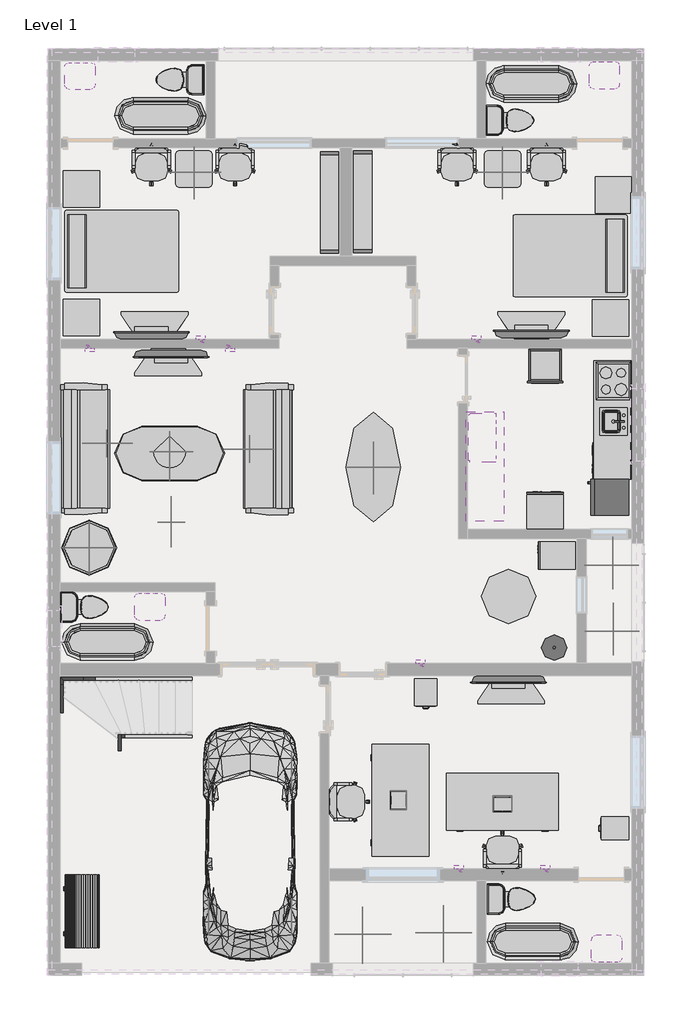
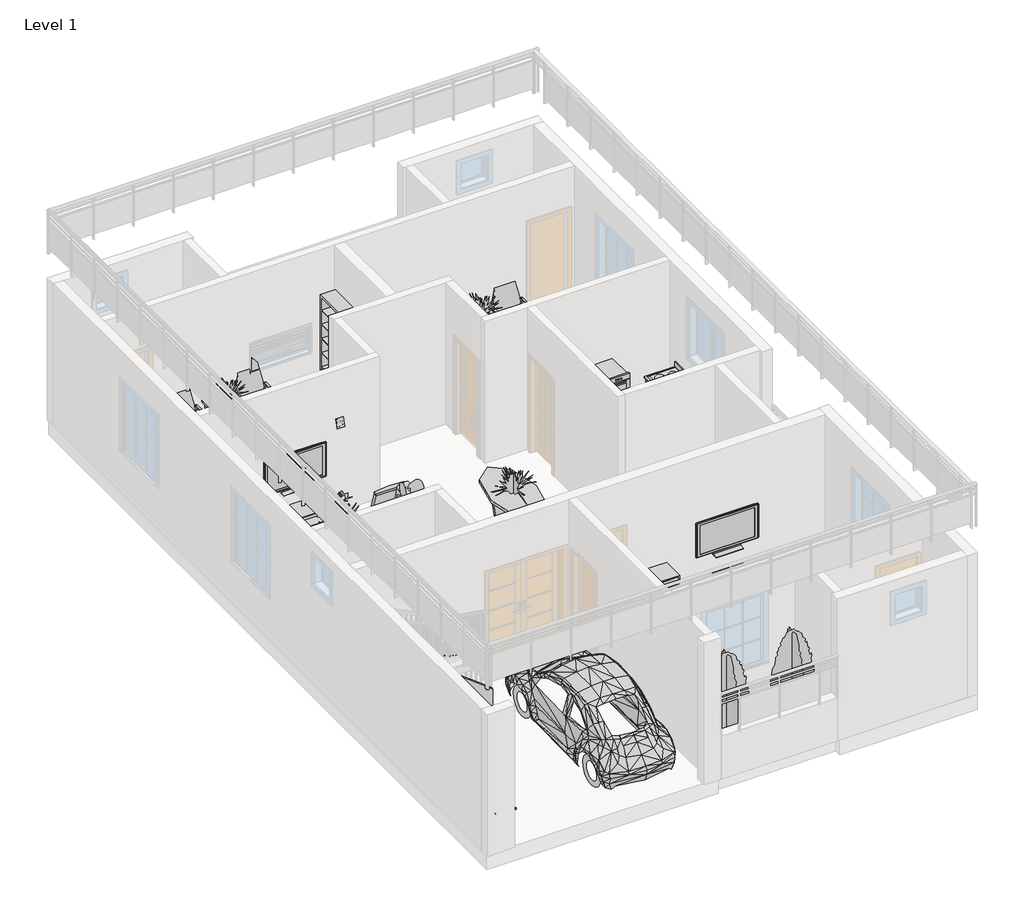
# One storey, part 5 of 5: 36 furniture elements, 22 proxies, 14 flow terminals, 10 geographic elements, 6 members.
"""IFC4 building model written with IfcOpenShell, lengths in millimetres."""

from ifc_helpers import new_model, si_unit, frame, origin, place, context, project, spatial, polyline, outline, extrude, triangles, transform, mapped, element, save
from components import entourage_4c8cfd20, proxy_7e1014cc, proxy_a6faaae8, proxy_45b28599, kitchenette_medium_kitchenette_medium_844211aa, proxy_5fdb4fb0, proxy_8b8c2dc4, rpc_beetle_rpc_beetle_3ce7ba48, rpc_female_69e001fa, rpc_picture_frame_rpc_picture_frame_c25e3fe9, proxy_c523a7b7, flow_terminal_871c2e40, flow_terminal_d49f872f, flow_terminal_62a433f7, toilet_domestic_3d_toilet_domestic_3d_f7549cf7, toilet_domestic_3d_toilet_domestic_3d_183bbd19, flow_terminal_2ffd2f66, furniture_0253826f, furniture_552c1472, chair_executive_chair_executive_8d69e98c, furniture_c6510c7c, furniture_d860a6bd, furniture_2fc54265, furniture_fcf97a65, furniture_aff9b2fb, furniture_fdf74506, tv_stand_tv_stand_6ce107e5, furniture_2c34a4f9, furniture_905aceb5, furniture_027a2ad9, furniture_bcf351fa, furniture_5bc9ed15, furniture_c80d6d9c, geographic_element_d8b57e58, rpc_plant_tropical_55f6ff97, rpc_plant_tropical_agave_1_5_93a2a214, rpc_plant_tropical_jungle_flame_3_9c4808c2, rpc_tree_conifer_chinese_juniper_7_1b9786cd

model = new_model("IFC4")

# Units and contexts
model_context = context("Model", 3, world=origin())
ifc_project = project(units=[si_unit("LENGTHUNIT", "METRE", prefix="MILLI")], contexts=[model_context])

# Site, building, storey
site = spatial("IfcSite", under=ifc_project)
building = spatial("IfcBuilding", under=site)
storey = spatial("IfcBuildingStorey", under=building, Name="Level 1", Elevation=0.0)

# Proxies
placement = place(None, origin())
element("IfcBuildingElementProxy", 1, Name="Building Element Proxy", at=placement, inside=storey, context=model_context, shape_type="Tessellation", body=[
    triangles([(-2574.7957443, 2173.9690475, 0.0), (-161.7957201, 2173.9690475, 0.0), (-187.195714, 802.3691202, 0.0), (-2549.3958412, 802.3691202, 0.0)], [[1, 4, 2], [3, 2, 4]], closed=False),
])
entourage_shape = entourage_4c8cfd20(model_context)
element("IfcBuildingElementProxy", 2, Name="Entourage", at=placement, inside=storey, context=model_context, shape_type="MappedRepresentation", body=[
    mapped(entourage_shape, transform((295.4042848, 3494.7691167, 762.0), x_axis=(1.0, 0.0, 0.0), y_axis=(0.0, 1.0, 0.0), z_axis=(0.0, 0.0, 1.0))),
])
element("IfcBuildingElementProxy", 3, Name="Entourage", at=placement, inside=storey, context=model_context, shape_type="MappedRepresentation", body=[
    mapped(entourage_shape, transform((-1406.3957152, 3520.1691167, 762.0), x_axis=(0.0, -1.0000000000000004, 0.0), y_axis=(1.0000000000000004, 0.0, 0.0), z_axis=(0.0, 0.0, 1.0))),
])
proxy_shape = proxy_7e1014cc(model_context)
element("IfcBuildingElementProxy", 4, Name="18\" x 24\" x 34 1/2\"", ObjectType="18\" x 24\" x 34 1/2\"", at=placement, inside=storey, context=model_context, shape_type="MappedRepresentation", body=[
    mapped(proxy_shape, transform((943.3547201, 7915.6865852, 0.0), x_axis=(0.0, -1.0000000000000007, 0.0), y_axis=(1.0000000000000007, 0.0, 0.0), z_axis=(0.0, 0.0, 1.0))),
])
proxy_2_shape = proxy_a6faaae8(model_context)
element("IfcBuildingElementProxy", 5, Name="Cook Top-4 Unit2 : 22\" x 20\"", ObjectType="Cook Top-4 Unit2 : 22\" x 20\"", at=placement, inside=storey, context=model_context, shape_type="MappedRepresentation", body=[
    mapped(proxy_2_shape, transform((2149.6042848, 10517.8691167, 0.0), x_axis=(0.0, -1.0000000000000004, 0.0), y_axis=(1.0000000000000004, 0.0, 0.0), z_axis=(0.0, 0.0, 1.0))),
])
proxy_3_shape = proxy_45b28599(model_context)
element("IfcBuildingElementProxy", 6, Name="Dishwasher : 24\" x 24\" x 34\"", ObjectType="Dishwasher : 24\" x 24\" x 34\"", at=placement, inside=storey, context=model_context, shape_type="MappedRepresentation", body=[
    mapped(proxy_3_shape, transform((1857.7547201, 9566.6865852, 0.0), x_axis=(0.0, -1.0000000000000004, 0.0), y_axis=(1.0000000000000004, 0.0, 0.0), z_axis=(0.0, 0.0, 1.0))),
])
element("IfcBuildingElementProxy", 7, Name="Dishwasher : 24\" x 24\" x 34\"", ObjectType="Dishwasher : 24\" x 24\" x 34\"", at=placement, inside=storey, context=model_context, shape_type="MappedRepresentation", body=[
    mapped(proxy_3_shape, transform((1388.9217533, 8612.6186815, 0.0), x_axis=(-1.0000000000000002, 0.0, 0.0), y_axis=(0.0, -1.0000000000000002, 0.0), z_axis=(0.0, 0.0, 1.0))),
])
kitchenette_medium_kitchenette_medium_shape = kitchenette_medium_kitchenette_medium_844211aa(model_context)
element("IfcBuildingElementProxy", 8, Name="Kitchenette - Medium : Kitchenette - Medium", ObjectType="Kitchenette - Medium : Kitchenette - Medium", at=placement, inside=storey, context=model_context, shape_type="MappedRepresentation", body=[
    mapped(kitchenette_medium_kitchenette_medium_shape, transform((2454.4042848, 10193.7068216, 0.0), x_axis=(0.0, -1.0000000000000004, 0.0), y_axis=(1.0000000000000004, 0.0, 0.0), z_axis=(0.0, 0.0, 1.0))),
])
proxy_4_shape = proxy_5fdb4fb0(model_context)
element("IfcBuildingElementProxy", 9, Name="Microwave : 32\" x 18\" x 20\"", ObjectType="Microwave : 32\" x 18\" x 20\"", at=placement, inside=storey, context=model_context, shape_type="MappedRepresentation", body=[
    mapped(proxy_4_shape, transform((-400.576221, 9073.7001436, 914.4), x_axis=(0.0, 1.0, 0.0), y_axis=(-1.0, 0.0, 0.0), z_axis=(0.0, 0.0, 1.0))),
])
proxy_5_shape = proxy_8b8c2dc4(model_context)
element("IfcBuildingElementProxy", 10, Name="Oven Double-Built-in : 21 1/2\" x 39 1/4\" x 21\"", ObjectType="Oven Double-Built-in : 21 1/2\" x 39 1/4\" x 21\"", at=placement, inside=storey, context=model_context, shape_type="MappedRepresentation", body=[
    mapped(proxy_5_shape, transform((1041.7792122, 10643.5032577, 0.0), x_axis=(1.0, 0.0, 0.0), y_axis=(0.0, 1.0, 0.0), z_axis=(0.0, 0.0, 1.0))),
])
rpc_beetle_rpc_beetle_shape = rpc_beetle_rpc_beetle_3ce7ba48(model_context)
element("IfcBuildingElementProxy", 11, Name="RPC Beetle : RPC Beetle", ObjectType="RPC Beetle : RPC Beetle", at=placement, inside=storey, context=model_context, shape_type="MappedRepresentation", body=[
    mapped(rpc_beetle_rpc_beetle_shape, transform((-3920.9957152, 1589.7691167, 0.0), x_axis=(1.0, 0.0, 0.0), y_axis=(0.0, 1.0, 0.0), z_axis=(0.0, 0.0, 1.0))),
])
rpc_female_shape = rpc_female_69e001fa(model_context)
element("IfcBuildingElementProxy", 12, Name="RPC Female", ObjectType="RPC Female", at=placement, inside=storey, context=model_context, shape_type="MappedRepresentation", body=[
    mapped(rpc_female_shape, transform((-5235.4778285, 8320.7691167, 0.0), x_axis=(-1.0000000000000004, 0.0, 0.0), y_axis=(0.0, -1.0000000000000004, 0.0), z_axis=(0.0, 0.0, 1.0))),
])
element("IfcBuildingElementProxy", 13, Name="RPC Female", ObjectType="RPC Female", at=placement, inside=storey, context=model_context, shape_type="MappedRepresentation", body=[
    mapped(rpc_female_shape, transform((-6156.1957152, 9474.3689452, 0.0), x_axis=(0.0, 1.0, 0.0), y_axis=(-1.0, 0.0, 0.0), z_axis=(0.0, 0.0, 1.0))),
])
element("IfcBuildingElementProxy", 14, Name="RPC Female", ObjectType="RPC Female", at=placement, inside=storey, context=model_context, shape_type="MappedRepresentation", body=[
    mapped(rpc_female_shape, transform((-4095.6217824, 9387.5691167, 0.0), x_axis=(0.0, -1.0000000000000002, 0.0), y_axis=(1.0000000000000002, 0.0, 0.0), z_axis=(0.0, 0.0, 1.0))),
])
rpc_picture_frame_rpc_picture_frame_shape = rpc_picture_frame_rpc_picture_frame_c25e3fe9(model_context)
element("IfcBuildingElementProxy", 15, Name="RPC Picture Frame : RPC Picture Frame", ObjectType="RPC Picture Frame : RPC Picture Frame", at=placement, inside=storey, context=model_context, shape_type="MappedRepresentation", body=[
    mapped(rpc_picture_frame_rpc_picture_frame_shape, transform((-1076.8648403, 5806.1691167, 1828.8), x_axis=(-1.0000000000000004, 0.0, 0.0), y_axis=(0.0, -1.0000000000000004, 0.0), z_axis=(0.0, 0.0, 1.0))),
])
element("IfcBuildingElementProxy", 16, Name="RPC Picture Frame : RPC Picture Frame", ObjectType="RPC Picture Frame : RPC Picture Frame", at=placement, inside=storey, context=model_context, shape_type="MappedRepresentation", body=[
    mapped(rpc_picture_frame_rpc_picture_frame_shape, transform((-4256.1312654, 11063.9691167, 1828.8), x_axis=(1.0000000000000002, 0.0, 0.0), y_axis=(0.0, 1.0000000000000002, 0.0), z_axis=(0.0, 0.0, 1.0))),
])
element("IfcBuildingElementProxy", 17, Name="RPC Picture Frame : RPC Picture Frame", ObjectType="RPC Picture Frame : RPC Picture Frame", at=placement, inside=storey, context=model_context, shape_type="MappedRepresentation", body=[
    mapped(rpc_picture_frame_rpc_picture_frame_shape, transform((-6603.3514055, 11063.9691167, 1828.8), x_axis=(1.0, 0.0, 0.0), y_axis=(0.0, 1.0, 0.0), z_axis=(0.0, 0.0, 1.0))),
])
element("IfcBuildingElementProxy", 18, Name="RPC Picture Frame : RPC Picture Frame", ObjectType="RPC Picture Frame : RPC Picture Frame", at=placement, inside=storey, context=model_context, shape_type="MappedRepresentation", body=[
    mapped(rpc_picture_frame_rpc_picture_frame_shape, transform((-142.9943815, 11216.3691167, 1828.8), x_axis=(-1.0, 0.0, 0.0), y_axis=(0.0, -1.0, 0.0), z_axis=(0.0, 0.0, 1.0))),
])
element("IfcBuildingElementProxy", 19, Name="RPC Picture Frame : RPC Picture Frame", ObjectType="RPC Picture Frame : RPC Picture Frame", at=placement, inside=storey, context=model_context, shape_type="MappedRepresentation", body=[
    mapped(rpc_picture_frame_rpc_picture_frame_shape, transform((-4752.5208659, 11216.3691167, 1828.8), x_axis=(-1.0, 0.0, 0.0), y_axis=(0.0, -1.0, 0.0), z_axis=(0.0, 0.0, 1.0))),
])
element("IfcBuildingElementProxy", 20, Name="RPC Picture Frame : RPC Picture Frame", ObjectType="RPC Picture Frame : RPC Picture Frame", at=placement, inside=storey, context=model_context, shape_type="MappedRepresentation", body=[
    mapped(rpc_picture_frame_rpc_picture_frame_shape, transform((1009.9817355, 2377.1691167, 1828.8), x_axis=(-1.0000000000000004, 0.0, 0.0), y_axis=(0.0, -1.0000000000000004, 0.0), z_axis=(0.0, 0.0, 1.0))),
])
element("IfcBuildingElementProxy", 21, Name="RPC Picture Frame : RPC Picture Frame", ObjectType="RPC Picture Frame : RPC Picture Frame", at=placement, inside=storey, context=model_context, shape_type="MappedRepresentation", body=[
    mapped(rpc_picture_frame_rpc_picture_frame_shape, transform((-433.5186179, 2377.1691167, 1828.8), x_axis=(-1.0, 0.0, 0.0), y_axis=(0.0, -1.0, 0.0), z_axis=(0.0, 0.0, 1.0))),
])
proxy_6_shape = proxy_c523a7b7(model_context)
element("IfcBuildingElementProxy", 22, Name="Refrigerator : 24\" x 25\" LH", ObjectType="Refrigerator : 24\" x 25\" LH", at=placement, inside=storey, context=model_context, shape_type="MappedRepresentation", body=[
    mapped(proxy_6_shape, transform((2103.9553134, 8581.1191167, 0.0), x_axis=(0.0, -1.0000000000000004, 0.0), y_axis=(1.0000000000000004, 0.0, 0.0), z_axis=(0.0, 0.0, 1.0))),
])

# Flow terminals
flow_terminal_shape = flow_terminal_871c2e40(model_context)
element("IfcFlowTerminal", 23, ObjectType="Sink Kitchen-Island : 18\" x 18\"", at=placement, inside=storey, context=model_context, shape_type="MappedRepresentation", body=[
    mapped(flow_terminal_shape, transform((2147.2588837, 9860.4583572, -14.4), x_axis=(0.0, -1.0000000000000004, 0.0), y_axis=(1.0000000000000004, 0.0, 0.0), z_axis=(0.0, 0.0, 1.0))),
])
flow_terminal_2_shape = flow_terminal_d49f872f(model_context)
element("IfcFlowTerminal", 24, ObjectType="Sink Vanity-Round : 19\" x 19\"", at=placement, inside=storey, context=model_context, shape_type="MappedRepresentation", body=[
    mapped(flow_terminal_2_shape, transform((1255.6560254, 6153.0886372, 609.6), x_axis=(-1.0, 0.0, 0.0), y_axis=(0.0, -1.0, 0.0), z_axis=(0.0, 0.0, 1.0))),
])
flow_terminal_3_shape = flow_terminal_62a433f7(model_context)
element("IfcFlowTerminal", 25, ObjectType="Sink Vanity-Square : 20\" x 18\"", at=placement, inside=storey, context=model_context, shape_type="MappedRepresentation", body=[
    mapped(flow_terminal_3_shape, transform((-5613.0849557, 6794.4237156, 914.4), x_axis=(1.0, 0.0, 0.0), y_axis=(0.0, 1.0, 0.0), z_axis=(0.0, 0.0, 1.0))),
])
element("IfcFlowTerminal", 26, ObjectType="Sink Vanity-Square : 20\" x 18\"", at=placement, inside=storey, context=model_context, shape_type="MappedRepresentation", body=[
    mapped(flow_terminal_3_shape, transform((-6781.4849557, 15659.0237156, 914.4), x_axis=(1.0, 0.0, 0.0), y_axis=(0.0, 1.0, 0.0), z_axis=(0.0, 0.0, 1.0))),
])
element("IfcFlowTerminal", 27, ObjectType="Sink Vanity-Square : 20\" x 18\"", at=placement, inside=storey, context=model_context, shape_type="MappedRepresentation", body=[
    mapped(flow_terminal_3_shape, transform((1981.5150443, 15671.7237156, 914.4), x_axis=(1.0, 0.0, 0.0), y_axis=(0.0, 1.0, 0.0), z_axis=(0.0, 0.0, 1.0))),
])
element("IfcFlowTerminal", 28, ObjectType="Sink Vanity-Square : 20\" x 18\"", at=placement, inside=storey, context=model_context, shape_type="MappedRepresentation", body=[
    mapped(flow_terminal_3_shape, transform((2050.9935254, 995.2145178, 914.4), x_axis=(-1.0, 0.0, 0.0), y_axis=(0.0, -1.0, 0.0), z_axis=(0.0, 0.0, 1.0))),
])
toilet_domestic_3d_toilet_domestic_3d_shape = toilet_domestic_3d_toilet_domestic_3d_f7549cf7(model_context)
toilet_domestic_3d_toilet_domestic_3d_2_shape = toilet_domestic_3d_toilet_domestic_3d_183bbd19(model_context)
element("IfcFlowTerminal", 29, ObjectType="Toilet-Domestic-3D : Toilet-Domestic-3D", at=placement, inside=storey, context=model_context, shape_type="MappedRepresentation", body=[
    mapped(toilet_domestic_3d_toilet_domestic_3d_shape, transform((-6601.2996878, 6745.9691167, 0.0), x_axis=(0.0, 1.0000000000000002, 0.0), y_axis=(-1.0000000000000002, 0.0, 0.0), z_axis=(0.0, 0.0, 1.0))),
    mapped(toilet_domestic_3d_toilet_domestic_3d_2_shape, transform((-6601.2996878, 6745.9691167, 0.0), x_axis=(0.0, 1.0000000000000002, 0.0), y_axis=(-1.0000000000000002, 0.0, 0.0), z_axis=(0.0, 0.0, 1.0))),
])
element("IfcFlowTerminal", 30, ObjectType="Toilet-Domestic-3D : Toilet-Domestic-3D", at=placement, inside=storey, context=model_context, shape_type="MappedRepresentation", body=[
    mapped(toilet_domestic_3d_toilet_domestic_3d_shape, transform((-5189.170729, 15552.2311807, 0.0), x_axis=(0.0, -1.0000000000000002, 0.0), y_axis=(1.0000000000000002, 0.0, 0.0), z_axis=(0.0, 0.0, 1.0))),
    mapped(toilet_domestic_3d_toilet_domestic_3d_2_shape, transform((-5189.170729, 15552.2311807, 0.0), x_axis=(0.0, -1.0000000000000002, 0.0), y_axis=(1.0000000000000002, 0.0, 0.0), z_axis=(0.0, 0.0, 1.0))),
])
element("IfcFlowTerminal", 31, ObjectType="Toilet-Domestic-3D : Toilet-Domestic-3D", at=placement, inside=storey, context=model_context, shape_type="MappedRepresentation", body=[
    mapped(toilet_domestic_3d_toilet_domestic_3d_shape, transform((510.7003122, 14873.9691167, 0.0), x_axis=(0.0, 1.0000000000000002, 0.0), y_axis=(-1.0000000000000002, 0.0, 0.0), z_axis=(0.0, 0.0, 1.0))),
    mapped(toilet_domestic_3d_toilet_domestic_3d_2_shape, transform((510.7003122, 14873.9691167, 0.0), x_axis=(0.0, 1.0000000000000002, 0.0), y_axis=(-1.0000000000000002, 0.0, 0.0), z_axis=(0.0, 0.0, 1.0))),
])
element("IfcFlowTerminal", 32, ObjectType="Toilet-Domestic-3D : Toilet-Domestic-3D", at=placement, inside=storey, context=model_context, shape_type="MappedRepresentation", body=[
    mapped(toilet_domestic_3d_toilet_domestic_3d_shape, transform((536.1003122, 1869.1691167, 0.0), x_axis=(0.0, 1.0000000000000002, 0.0), y_axis=(-1.0000000000000002, 0.0, 0.0), z_axis=(0.0, 0.0, 1.0))),
    mapped(toilet_domestic_3d_toilet_domestic_3d_2_shape, transform((536.1003122, 1869.1691167, 0.0), x_axis=(0.0, 1.0000000000000002, 0.0), y_axis=(-1.0000000000000002, 0.0, 0.0), z_axis=(0.0, 0.0, 1.0))),
])
flow_terminal_4_shape = flow_terminal_2ffd2f66(model_context)
element("IfcFlowTerminal", 33, ObjectType="Tub-Free Standing-3D : 30\" x 60\"", at=placement, inside=storey, context=model_context, shape_type="MappedRepresentation", body=[
    mapped(flow_terminal_4_shape, transform((-6308.5957152, 6161.7691167, 0.0), x_axis=(0.0, 1.0000000000000002, 0.0), y_axis=(-1.0000000000000002, 0.0, 0.0), z_axis=(0.0, 0.0, 1.0))),
])
element("IfcFlowTerminal", 34, ObjectType="Tub-Free Standing-3D : 30\" x 60\"", at=placement, inside=storey, context=model_context, shape_type="MappedRepresentation", body=[
    mapped(flow_terminal_4_shape, transform((-5419.5957152, 14950.1691167, 0.0), x_axis=(0.0, -1.0000000000000004, 0.0), y_axis=(1.0000000000000004, 0.0, 0.0), z_axis=(0.0, 0.0, 1.0))),
])
element("IfcFlowTerminal", 35, ObjectType="Tub-Free Standing-3D : 30\" x 60\"", at=placement, inside=storey, context=model_context, shape_type="MappedRepresentation", body=[
    mapped(flow_terminal_4_shape, transform((778.0042848, 15483.5691167, 0.0), x_axis=(0.0, 1.0000000000000002, 0.0), y_axis=(-1.0000000000000002, 0.0, 0.0), z_axis=(0.0, 0.0, 1.0))),
])
element("IfcFlowTerminal", 36, ObjectType="Tub-Free Standing-3D : 30\" x 60\"", at=placement, inside=storey, context=model_context, shape_type="MappedRepresentation", body=[
    mapped(flow_terminal_4_shape, transform((803.4042848, 1157.9691167, 0.0), x_axis=(0.0, 1.0000000000000002, 0.0), y_axis=(-1.0000000000000002, 0.0, 0.0), z_axis=(0.0, 0.0, 1.0))),
])

# Furniture
furniture_shape = furniture_0253826f(model_context)
element("IfcFurniture", 37, ObjectType="Bed-Standard.0001 : Double 54\" x 75\"", at=placement, inside=storey, context=model_context, shape_type="MappedRepresentation", body=[
    mapped(furniture_shape, transform((-6112.8907971, 12418.0805921, 0.0), x_axis=(0.0, 1.0, 0.0), y_axis=(-1.0, 0.0, 0.0), z_axis=(0.0, 0.0, 1.0))),
])
element("IfcFurniture", 38, ObjectType="Bed-Standard.0001 : Double 54\" x 75\"", at=placement, inside=storey, context=model_context, shape_type="MappedRepresentation", body=[
    mapped(furniture_shape, transform((1471.2993668, 12884.8576413, 0.0), x_axis=(0.0, -1.0000000000000002, 0.0), y_axis=(1.0000000000000002, 0.0, 0.0), z_axis=(0.0, 0.0, 1.0))),
])
furniture_2_shape = furniture_552c1472(model_context)
element("IfcFurniture", 39, ObjectType="Cabinet-File 3 Drawer.0001 : 15\" x 18\"", at=placement, inside=storey, context=model_context, shape_type="MappedRepresentation", body=[
    mapped(furniture_2_shape, transform((-859.3992681, 5465.7034168, 0.0), x_axis=(1.0, 0.0, 0.0), y_axis=(0.0, 1.0, 0.0), z_axis=(0.0, 0.0, 1.0))),
])
element("IfcFurniture", 40, ObjectType="Cabinet-File 3 Drawer.0001 : 15\" x 18\"", at=placement, inside=storey, context=model_context, shape_type="MappedRepresentation", body=[
    mapped(furniture_2_shape, transform((2317.138585, 2922.3726696, 0.0), x_axis=(0.0, -1.0000000000000004, 0.0), y_axis=(1.0000000000000004, 0.0, 0.0), z_axis=(0.0, 0.0, 1.0))),
])
chair_executive_chair_executive_shape = chair_executive_chair_executive_8d69e98c(model_context)
element("IfcFurniture", 41, ObjectType="Chair-Executive : Chair-Executive", at=placement, inside=storey, context=model_context, shape_type="MappedRepresentation", body=[
    mapped(chair_executive_chair_executive_shape, transform((-5431.0048955, 14144.2398663, 0.0), x_axis=(-1.0000000000000004, 0.0, 0.0), y_axis=(0.0, -1.0000000000000004, 0.0), z_axis=(0.0, 0.0, 1.0))),
])
element("IfcFurniture", 42, ObjectType="Chair-Executive : Chair-Executive", at=placement, inside=storey, context=model_context, shape_type="MappedRepresentation", body=[
    mapped(chair_executive_chair_executive_shape, transform((-4034.0048955, 14144.2398663, 0.0), x_axis=(-1.0, 0.0, 0.0), y_axis=(0.0, -1.0, 0.0), z_axis=(0.0, 0.0, 1.0))),
])
element("IfcFurniture", 43, ObjectType="Chair-Executive : Chair-Executive", at=placement, inside=storey, context=model_context, shape_type="MappedRepresentation", body=[
    mapped(chair_executive_chair_executive_shape, transform((1172.9951045, 14144.2398663, 0.0), x_axis=(-0.9999999999999998, 0.0, 0.0), y_axis=(0.0, -0.9999999999999998, 0.0), z_axis=(0.0, 0.0, 1.0))),
])
element("IfcFurniture", 44, ObjectType="Chair-Executive : Chair-Executive", at=placement, inside=storey, context=model_context, shape_type="MappedRepresentation", body=[
    mapped(chair_executive_chair_executive_shape, transform((-322.4309627, 14144.2398663, 0.0), x_axis=(-1.0, 0.0, 0.0), y_axis=(0.0, -1.0, 0.0), z_axis=(0.0, 0.0, 1.0))),
])
element("IfcFurniture", 45, ObjectType="Chair-Executive : Chair-Executive", at=placement, inside=storey, context=model_context, shape_type="MappedRepresentation", body=[
    mapped(chair_executive_chair_executive_shape, transform((-2288.9416168, 3635.7599363, 0.0), x_axis=(0.0, -1.0000000000000007, 0.0), y_axis=(1.0000000000000007, 0.0, 0.0), z_axis=(0.0, 0.0, 1.0))),
])
element("IfcFurniture", 46, ObjectType="Chair-Executive : Chair-Executive", at=placement, inside=storey, context=model_context, shape_type="MappedRepresentation", body=[
    mapped(chair_executive_chair_executive_shape, transform((154.4134652, 2637.623215, 0.0), x_axis=(1.0000000000000009, 0.0, 0.0), y_axis=(0.0, 1.0000000000000009, 0.0), z_axis=(0.0, 0.0, 1.0))),
])
furniture_3_shape = furniture_c6510c7c(model_context)
element("IfcFurniture", 47, ObjectType="Counter Top w Sink Hole : 24\" Depth", at=placement, inside=storey, context=model_context, shape_type="MappedRepresentation", body=[
    mapped(furniture_3_shape, transform((2454.4042848, 9660.3068216, -14.4), x_axis=(0.0, -1.0000000000000004, 0.0), y_axis=(1.0000000000000004, 0.0, 0.0), z_axis=(0.0, 0.0, 1.0))),
])
furniture_4_shape = furniture_d860a6bd(model_context)
element("IfcFurniture", 48, ObjectType="Counter Top w Sink Hole : 24\" Depth", at=placement, inside=storey, context=model_context, shape_type="MappedRepresentation", body=[
    mapped(furniture_4_shape, transform((320.8042848, 9377.455316, 914.4), x_axis=(0.0, 1.0000000000000002, 0.0), y_axis=(-1.0000000000000002, 0.0, 0.0), z_axis=(0.0, 0.0, 1.0))),
])
furniture_5_shape = furniture_2fc54265(model_context)
element("IfcFurniture", 49, ObjectType="Desk : 72\" x 36\"", at=placement, inside=storey, context=model_context, shape_type="MappedRepresentation", body=[
    mapped(furniture_5_shape, transform((-949.1957152, 2605.7691167, 0.0), x_axis=(0.0, 1.000000000000001, 0.0), y_axis=(-1.000000000000001, 0.0, 0.0), z_axis=(0.0, 0.0, 1.0))),
])
element("IfcFurniture", 50, ObjectType="Desk : 72\" x 36\"", at=placement, inside=storey, context=model_context, shape_type="MappedRepresentation", body=[
    mapped(furniture_5_shape, transform((1209.8042848, 3951.9691167, 0.0), x_axis=(-1.0000000000000022, 0.0, 0.0), y_axis=(0.0, -1.0000000000000022, 0.0), z_axis=(0.0, 0.0, 1.0))),
])
furniture_6_shape = furniture_fcf97a65(model_context)
element("IfcFurniture", 51, ObjectType="Shelving : 96\" x 12\" x 84\"", at=placement, inside=storey, context=model_context, shape_type="MappedRepresentation", body=[
    mapped(furniture_6_shape, transform((-2901.8217824, 13502.3691167, 0.0), x_axis=(0.0, 1.0, 0.0), y_axis=(-1.0, 0.0, 0.0), z_axis=(0.0, 0.0, 1.0))),
])
element("IfcFurniture", 52, ObjectType="Shelving : 96\" x 12\" x 84\"", at=placement, inside=storey, context=model_context, shape_type="MappedRepresentation", body=[
    mapped(furniture_6_shape, transform((-2346.1957152, 13515.6939646, 0.0), x_axis=(0.0, 1.0, 0.0), y_axis=(-1.0, 0.0, 0.0), z_axis=(0.0, 0.0, 1.0))),
])
furniture_7_shape = furniture_aff9b2fb(model_context)
element("IfcFurniture", 53, ObjectType="Sofa-Pensi : 84\"", at=placement, inside=storey, context=model_context, shape_type="MappedRepresentation", body=[
    mapped(furniture_7_shape, transform((-6412.4858791, 9108.9628667, 0.0), x_axis=(0.0, 1.0000000000000002, 0.0), y_axis=(-1.0000000000000002, 0.0, 0.0), z_axis=(0.0, 0.0, 1.0))),
])
element("IfcFurniture", 54, ObjectType="Sofa-Pensi : 84\"", at=placement, inside=storey, context=model_context, shape_type="MappedRepresentation", body=[
    mapped(furniture_7_shape, transform((-3893.3055512, 9666.1753667, 0.0), x_axis=(0.0, -1.0000000000000007, 0.0), y_axis=(1.0000000000000007, 0.0, 0.0), z_axis=(0.0, 0.0, 1.0))),
])
furniture_8_shape = furniture_fdf74506(model_context)
element("IfcFurniture", 55, ObjectType="TV - Flat Screen : 50\"", at=placement, inside=storey, context=model_context, shape_type="MappedRepresentation", body=[
    mapped(furniture_8_shape, transform((-5575.9402293, 11274.9077403, 914.4), x_axis=(-1.0000000000000002, 0.0, 0.0), y_axis=(0.0, -1.0000000000000002, 0.0), z_axis=(0.0, 0.0, 1.0))),
])
element("IfcFurniture", 56, ObjectType="TV - Flat Screen : 50\"", at=placement, inside=storey, context=model_context, shape_type="MappedRepresentation", body=[
    mapped(furniture_8_shape, transform((774.0597707, 11300.3077403, 914.4), x_axis=(-1.0, 0.0, 0.0), y_axis=(0.0, -1.0, 0.0), z_axis=(0.0, 0.0, 1.0))),
])
element("IfcFurniture", 57, ObjectType="TV - Flat Screen : 50\"", at=placement, inside=storey, context=model_context, shape_type="MappedRepresentation", body=[
    mapped(furniture_8_shape, transform((-5239.0042172, 10980.030493, 914.4), x_axis=(1.0000000000000007, 0.0, 0.0), y_axis=(0.0, 1.0000000000000007, 0.0), z_axis=(0.0, 0.0, 1.0))),
])
element("IfcFurniture", 58, ObjectType="TV - Flat Screen : 50\"", at=placement, inside=storey, context=model_context, shape_type="MappedRepresentation", body=[
    mapped(furniture_8_shape, transform((399.3870585, 5544.8392173, 914.4), x_axis=(1.0000000000000007, 0.0, 0.0), y_axis=(0.0, 1.0000000000000007, 0.0), z_axis=(0.0, 0.0, 1.0))),
])
tv_stand_tv_stand_shape = tv_stand_tv_stand_6ce107e5(model_context)
element("IfcFurniture", 59, ObjectType="TV Stand : TV Stand", at=placement, inside=storey, context=model_context, shape_type="MappedRepresentation", body=[
    mapped(tv_stand_tv_stand_shape, transform((-5396.0077131, 11216.3691167, 0.0), x_axis=(-1.0000000000000004, 0.0, 0.0), y_axis=(0.0, -1.0000000000000004, 0.0), z_axis=(0.0, 0.0, 1.0))),
])
element("IfcFurniture", 60, ObjectType="TV Stand : TV Stand", at=placement, inside=storey, context=model_context, shape_type="MappedRepresentation", body=[
    mapped(tv_stand_tv_stand_shape, transform((903.1922869, 11216.3691167, 0.0), x_axis=(-1.0, 0.0, 0.0), y_axis=(0.0, -1.0, 0.0), z_axis=(0.0, 0.0, 1.0))),
])
element("IfcFurniture", 61, ObjectType="TV Stand : TV Stand", at=placement, inside=storey, context=model_context, shape_type="MappedRepresentation", body=[
    mapped(tv_stand_tv_stand_shape, transform((-5414.6097845, 11063.9691167, 0.0), x_axis=(1.0000000000000009, 0.0, 0.0), y_axis=(0.0, 1.0000000000000009, 0.0), z_axis=(0.0, 0.0, 1.0))),
])
element("IfcFurniture", 62, ObjectType="TV Stand : TV Stand", at=placement, inside=storey, context=model_context, shape_type="MappedRepresentation", body=[
    mapped(tv_stand_tv_stand_shape, transform((314.7936208, 5588.5657114, 0.0), x_axis=(1.0000000000000009, 0.0, 0.0), y_axis=(0.0, 1.0000000000000009, 0.0), z_axis=(0.0, 0.0, 1.0))),
])
furniture_9_shape = furniture_2c34a4f9(model_context)
element("IfcFurniture", 63, ObjectType="Table-Dining Oval : 36\" x 72\"", at=placement, inside=storey, context=model_context, shape_type="MappedRepresentation", body=[
    mapped(furniture_9_shape, transform((-5669.0153873, 8953.270756, 0.0), x_axis=(-1.0000000000000002, 0.0, 0.0), y_axis=(0.0, -1.0000000000000002, 0.0), z_axis=(0.0, 0.0, 1.0))),
])
furniture_10_shape = furniture_905aceb5(model_context)
element("IfcFurniture", 64, ObjectType="Table-Dining Round w Chairs : 36\" Diameter", at=placement, inside=storey, context=model_context, shape_type="MappedRepresentation", body=[
    mapped(furniture_10_shape, transform((293.3223176, 7108.6478052, 0.0), x_axis=(1.0, 0.0, 0.0), y_axis=(0.0, 1.0, 0.0), z_axis=(0.0, 0.0, 1.0))),
])
furniture_11_shape = furniture_027a2ad9(model_context)
element("IfcFurniture", 65, ObjectType="Table-Ellipse : 72\" x 36\"", at=placement, inside=storey, context=model_context, shape_type="MappedRepresentation", body=[
    mapped(furniture_11_shape, transform((-1863.5957152, 9082.7691167, 0.0), x_axis=(0.0, 1.0000000000000002, 0.0), y_axis=(-1.0000000000000002, 0.0, 0.0), z_axis=(0.0, 0.0, 1.0))),
])
furniture_12_shape = furniture_bcf351fa(model_context)
element("IfcFurniture", 66, ObjectType="Table-End : 24\" x 24\"", at=placement, inside=storey, context=model_context, shape_type="MappedRepresentation", body=[
    mapped(furniture_12_shape, transform((-5169.3293454, 13908.7691167, 0.0), x_axis=(1.0, 0.0, 0.0), y_axis=(0.0, 1.0, 0.0), z_axis=(0.0, 0.0, 1.0))),
])
element("IfcFurniture", 67, ObjectType="Table-End : 24\" x 24\"", at=placement, inside=storey, context=model_context, shape_type="MappedRepresentation", body=[
    mapped(furniture_12_shape, transform((-13.1293454, 13908.7691167, 0.0), x_axis=(1.0, 0.0, 0.0), y_axis=(0.0, 1.0, 0.0), z_axis=(0.0, 0.0, 1.0))),
])
furniture_13_shape = furniture_5bc9ed15(model_context)
element("IfcFurniture", 68, ObjectType="Table-Night Stand : 24\" x 24\" x 30\"", at=placement, inside=storey, context=model_context, shape_type="MappedRepresentation", body=[
    mapped(furniture_13_shape, transform((-7048.9293454, 11280.4939646, 0.0), x_axis=(1.0, 0.0, 0.0), y_axis=(0.0, 1.0, 0.0), z_axis=(0.0, 0.0, 1.0))),
])
element("IfcFurniture", 69, ObjectType="Table-Night Stand : 24\" x 24\" x 30\"", at=placement, inside=storey, context=model_context, shape_type="MappedRepresentation", body=[
    mapped(furniture_13_shape, transform((-7048.9293454, 13426.1691167, 0.0), x_axis=(1.0, 0.0, 0.0), y_axis=(0.0, 1.0, 0.0), z_axis=(0.0, 0.0, 1.0))),
])
element("IfcFurniture", 70, ObjectType="Table-Night Stand : 24\" x 24\" x 30\"", at=placement, inside=storey, context=model_context, shape_type="MappedRepresentation", body=[
    mapped(furniture_13_shape, transform((1790.2706546, 11267.1691167, 0.0), x_axis=(1.0, 0.0, 0.0), y_axis=(0.0, 1.0, 0.0), z_axis=(0.0, 0.0, 1.0))),
])
element("IfcFurniture", 71, ObjectType="Table-Night Stand : 24\" x 24\" x 30\"", at=placement, inside=storey, context=model_context, shape_type="MappedRepresentation", body=[
    mapped(furniture_13_shape, transform((1841.0706546, 13324.5691167, 0.0), x_axis=(1.0, 0.0, 0.0), y_axis=(0.0, 1.0, 0.0), z_axis=(0.0, 0.0, 1.0))),
])
furniture_14_shape = furniture_c80d6d9c(model_context)
element("IfcFurniture", 72, ObjectType="Table-Round : 36\" Diameter", at=placement, inside=storey, context=model_context, shape_type="MappedRepresentation", body=[
    mapped(furniture_14_shape, transform((-6613.3957152, 7736.5691167, 0.0), x_axis=(1.0, 0.0, 0.0), y_axis=(0.0, 1.0, 0.0), z_axis=(0.0, 0.0, 1.0))),
])

# Geographic elements
geographic_element_shape = geographic_element_d8b57e58(model_context)
element("IfcGeographicElement", 73, ObjectType="Park Bench : 72\"", at=placement, inside=storey, context=model_context, shape_type="MappedRepresentation", body=[
    mapped(geographic_element_shape, transform((-6765.7957152, 1665.9691167, 0.0), x_axis=(0.0, 1.0000000000000002, 0.0), y_axis=(-1.0000000000000002, 0.0, 0.0), z_axis=(0.0, 0.0, 1.0))),
])
rpc_plant_tropical_shape = rpc_plant_tropical_55f6ff97(model_context)
element("IfcGeographicElement", 74, ObjectType="RPC Plant - Tropical", at=placement, inside=storey, context=model_context, shape_type="MappedRepresentation", body=[
    mapped(rpc_plant_tropical_shape, transform((-5267.1957152, 9336.7691167, 914.4), x_axis=(1.0, 0.0, 0.0), y_axis=(0.0, 1.0, 0.0), z_axis=(0.0, 0.0, 1.0))),
])
rpc_plant_tropical_agave_1_5_shape = rpc_plant_tropical_agave_1_5_93a2a214(model_context)
element("IfcGeographicElement", 75, ObjectType="RPC Plant - Tropical : Agave - 1.5'", at=placement, inside=storey, context=model_context, shape_type="MappedRepresentation", body=[
    mapped(rpc_plant_tropical_agave_1_5_shape, transform((-4860.7957152, 14010.3691167, 762.0), x_axis=(1.0, 0.0, 0.0), y_axis=(0.0, 1.0, 0.0), z_axis=(0.0, 0.0, 1.0))),
])
element("IfcGeographicElement", 76, ObjectType="RPC Plant - Tropical : Agave - 1.5'", at=placement, inside=storey, context=model_context, shape_type="MappedRepresentation", body=[
    mapped(rpc_plant_tropical_agave_1_5_shape, transform((295.4042848, 14010.3691167, 762.0), x_axis=(1.0, 0.0, 0.0), y_axis=(0.0, 1.0, 0.0), z_axis=(0.0, 0.0, 1.0))),
])
element("IfcGeographicElement", 77, ObjectType="RPC Plant - Tropical : Agave - 1.5'", at=placement, inside=storey, context=model_context, shape_type="MappedRepresentation", body=[
    mapped(rpc_plant_tropical_agave_1_5_shape, transform((-6613.3957152, 7736.5691167, 762.0), x_axis=(1.0, 0.0, 0.0), y_axis=(0.0, 1.0, 0.0), z_axis=(0.0, 0.0, 1.0))),
])
element("IfcGeographicElement", 78, ObjectType="RPC Plant - Tropical : Agave - 1.5'", at=placement, inside=storey, context=model_context, shape_type="MappedRepresentation", body=[
    mapped(rpc_plant_tropical_agave_1_5_shape, transform((-1863.5957152, 9082.7691167, 762.0), x_axis=(1.0, 0.0, 0.0), y_axis=(0.0, 1.0, 0.0), z_axis=(0.0, 0.0, 1.0))),
])
rpc_plant_tropical_jungle_flame_3_shape = rpc_plant_tropical_jungle_flame_3_9c4808c2(model_context)
element("IfcGeographicElement", 79, ObjectType="RPC Plant - Tropical : Jungle Flame - 3'", at=placement, inside=storey, context=model_context, shape_type="MappedRepresentation", body=[
    mapped(rpc_plant_tropical_jungle_flame_3_shape, transform((2149.6042848, 6339.5691167, 0.0), x_axis=(1.0, 0.0, 0.0), y_axis=(0.0, 1.0, 0.0), z_axis=(0.0, 0.0, 1.0))),
])
element("IfcGeographicElement", 80, ObjectType="RPC Plant - Tropical : Jungle Flame - 3'", at=placement, inside=storey, context=model_context, shape_type="MappedRepresentation", body=[
    mapped(rpc_plant_tropical_jungle_flame_3_shape, transform((2140.6907636, 7440.6995846, 0.0), x_axis=(1.0, 0.0, 0.0), y_axis=(0.0, 1.0, 0.0), z_axis=(0.0, 0.0, 1.0))),
])
rpc_tree_conifer_chinese_juniper_7_shape = rpc_tree_conifer_chinese_juniper_7_1b9786cd(model_context)
element("IfcGeographicElement", 81, ObjectType="RPC Tree - Conifer : Chinese Juniper - 7'", at=placement, inside=storey, context=model_context, shape_type="MappedRepresentation", body=[
    mapped(rpc_tree_conifer_chinese_juniper_7_shape, transform((-2041.5923862, 1284.9691167, 0.0), x_axis=(1.0, 0.0, 0.0), y_axis=(0.0, 1.0, 0.0), z_axis=(0.0, 0.0, 1.0))),
])
element("IfcGeographicElement", 82, ObjectType="RPC Tree - Conifer : Chinese Juniper - 7'", at=placement, inside=storey, context=model_context, shape_type="MappedRepresentation", body=[
    mapped(rpc_tree_conifer_chinese_juniper_7_shape, transform((-695.3923862, 1310.3691167, 0.0), x_axis=(1.0, 0.0, 0.0), y_axis=(0.0, 1.0, 0.0), z_axis=(0.0, 0.0, 1.0))),
])

# Members
element("IfcMember", 83, ObjectType="Stringer - 2\" Width", at=placement, inside=storey, context=model_context, shape_type="SweptSolid", body=[
    extrude(outline(polyline([(0.0, -4892.6027934), (354.8499298, -4892.6027934), (1254.5507317, -6079.9957152), (872.1359024, -6079.9957152), (0.0, -4928.9819614), (0.0, -4892.6027934)])), frame((0.0, 4561.5691167, 0.0), z_axis=(0.0, 1.0, 0.0), x_axis=(0.0, 0.0, 1.0)), (0.0, 0.0, 1.0), 50.8),
])
element("IfcMember", 84, ObjectType="Stringer - 2\" Width", at=placement, inside=storey, context=model_context, shape_type="SweptSolid", body=[
    extrude(outline(polyline([(4612.3691167, 1386.2105893), (4612.3691167, 1011.3402593), (2646.197182, 2419.0812849), (2646.197182, 2793.9516149), (4612.3691167, 1386.2105893)])), frame((-6130.7957152, 0.0, 0.0), z_axis=(1.0, 0.0, 0.0), x_axis=(0.0, 1.0, 0.0)), (0.0, 0.0, 1.0), 50.8),
])
element("IfcMember", 85, ObjectType="Stringer - 2\" Width", at=placement, inside=storey, context=model_context, shape_type="SweptSolid", body=[
    extrude(outline(polyline([(62.87986, -4892.6027934), (403.0231656, -4892.6027934), (1303.4198838, -6710.3543004), (963.2765782, -6710.3543004), (62.87986, -4892.6027934)])), frame((0.0, 5526.7691167, 0.0), z_axis=(0.0, 1.0, 0.0), x_axis=(0.0, 0.0, 1.0)), (0.0, 0.0, 1.0), 50.8),
])
element("IfcMember", 86, ObjectType="Stringer - 2\" Width", at=placement, inside=storey, context=model_context, shape_type="SweptSolid", body=[
    extrude(outline(polyline([(-6710.3543004, 5577.5691167), (-6710.3543004, 5526.7691167), (-7045.1957152, 5526.7691167), (-7095.9957152, 5577.5691167), (-6710.3543004, 5577.5691167)])), frame((0.0, 0.0, 963.2765782), z_axis=(0.0, 0.0, 1.0), x_axis=(1.0, 0.0, 0.0)), (0.0, 0.0, 1.0), 340.1433056),
])
element("IfcMember", 87, ObjectType="Stringer - 2\" Width", at=placement, inside=storey, context=model_context, shape_type="SweptSolid", body=[
    extrude(outline(polyline([(-7095.9957152, 5577.5691167), (-7045.1957152, 5526.7691167), (-7045.1957152, 5448.1728963), (-7095.9957152, 5448.1728963), (-7095.9957152, 5577.5691167)])), frame((0.0, 0.0, 963.2765782), z_axis=(0.0, 0.0, 1.0), x_axis=(1.0, 0.0, 0.0)), (0.0, 0.0, 1.0), 340.1433056),
])
element("IfcMember", 88, ObjectType="Stringer - 2\" Width", at=placement, inside=storey, context=model_context, shape_type="SweptSolid", body=[
    extrude(outline(polyline([(5448.1728963, 1303.4198838), (5448.1728963, 963.2765782), (2646.197182, 2373.9415335), (2646.197182, 2714.0848391), (5448.1728963, 1303.4198838)])), frame((-7095.9957152, 0.0, 0.0), z_axis=(1.0, 0.0, 0.0), x_axis=(0.0, 1.0, 0.0)), (0.0, 0.0, 1.0), 50.8),
])

save(model, "model.ifc")

# Revit data of these elements
# Type
#   built-in parameter 1005195 = "RPC-16-N04H-AQSP-D1N4-43SU-6GKQ-C3KU-1C"
#   Height = 0
# Type "18\" x 24\" x 34 1/2\""
#   Label = "T"
#   Assembly Code = "E1090400"
#   Depth = 2' - 0"
#   Height = 2' - 10 1/2"
#   Width = 1' - 6"
#   Panel Face Material = Plastic, Opaque Black
#   Trach Compact. Material = Steel, Paint Finish, Ivory, Matte
#   Default Elevation = 0
# Type "Cook Top-4 Unit2 : 22\" x 20\""
#   Depth = 1' - 8"
#   Width = 1' - 10"
#   Burner Material = Steel, Chrome Plated
#   Cooktop Material = Steel, Polished
#   Default Elevation = 0
#   Assembly Code = ""
# Type "Dishwasher : 24\" x 24\" x 34\""
#   Label = "DW"
#   Assembly Code = "E1090400"
#   Depth = 2' - 0"
#   Height = 2' - 10"
#   Width = 2' - 0"
#   Dishwasher Material = Steel, Paint Finish, Ivory, Glossy
#   Panel Face Material = Plastic, Opaque Black
#   Default Elevation = 0
# Type "Kitchenette - Medium : Kitchenette - Medium"
#   Assembly Code = "E1090400"
#   Counter Length = 6' - 6"
#   Cabinet Width = 4' - 6"
#   Cabinet Height = 2' - 10 1/2"
#   Cabinet Depth = 2' - 0"
#   Toe Depth = 0' - 3"
#   Toe Height = 0' - 3 1/2"
#   Cabinet Material = Cabinets
#   Door/Drawer Material = Cabinets
#   Handle Material = Cabinets - Handles
#   Default Elevation = 0
# Type "Microwave : 32\" x 18\" x 20\""
#   Assembly Code = "E1090400"
#   Depth = 1' - 6"
#   Height = 1' - 8"
#   Width = 2' - 8"
#   Microwave Material = Laminate, Ivory, Matte
#   Default Elevation = 0
# Type "Oven Double-Built-in : 21 1/2\" x 39 1/4\" x 21\""
#   Label = "OVEN"
#   Assembly Code = "E1090400"
#   Depth = 1' - 9"
#   Height = 3' - 3 1/4"
#   Width = 1' - 9 1/2"
#   Oven Material = Metal - Stainless Steel, Polished
#   Default Elevation = 0
# Type "RPC Beetle : RPC Beetle"
#   built-in parameter 1005195 = "RPC-16-0U6E-L4EG-ENH1-J3KF-SVEL-0TX4-C0"
#   Height = 0
# Type "RPC Female"
#   built-in parameter 1005195 = "RPC-8-FXA2-QQQ0-UGV2-6"
#   Height = 0
# Type "RPC Picture Frame : RPC Picture Frame"
#   built-in parameter 1005198 = "{2, 15},{39, RPC-16-8M5E-0H3T-F0AH-3U0K-JLQ7-G28B-AU},{1, 0},{1, 0},{2, 19},{1, 8},{5, Color},{1, 0},{1, 0},{3, 0.8},{3, 0.8},{3, 0.8},{1, 8},{7, BBoxMin},{1, 0},{1, 0},{1, 0},{1, 0},{1, 0},{1, 8},{7, BBoxMax},{1, 0},{1, 0},{1, 0},{1, 0},{1, 0},{2, 11},{9, RPCTypeId},{1, 0},{1, 0},{39, RPC-16-8M5E-0H3T-F0AH-3U0K-JLQ7-G28B-AU},{1, 6},{14, RPCPlantHeight},{1, 0},{1, 0},{5, 0.625},{2, 11},{7, keyword},{1, 0},{1, 0},{33, :RPCs:Office Clutter:Geometry:RPC},{2, 11},{8, category},{1, 0},{1, 0},{14, Office Clutter},{2, 11},{12, LocalizedUID},{1, 0},{1, 0},{13, Picture Frame},{2, 14},{6, Height},{1, 0},{1, 0},{5, 0.625},{1, 2},{16, Cast Reflections},{1, 0},{1, 0},{1, 0},{1, 2},{8, Portrait},{1, 0},{1, 0},{1, 1},{1, 2},{5, Stand},{1, 0},{1, 0},{1, 1},{2, 11},{10, RPCL_Frame},{1, 0},{1, 0},{5, Frame},{1, 4},{14, Frame Material},{1, 0},{1, 0},{1, 0},{2, 11},{12, RPCL_Picture},{1, 0},{1, 0},{7, Picture},{2, 11},{15, Picture Preview},{1, 0},{1, 0},{65, __RPC:/object data/textures/object/Photo/Photo0/textures/Portrait},{2, 11},{17, i_Picture Preview},{1, 0},{1, 0},{0, },{1, 2},{18, Use Custom Picture},{1, 0},{1, 0},{1, 0},{2, 11},{17, Picture File Name},{1, 0},{1, 0},{0, },{21, assetlibrary_base.fbx},{1, 5},"
#   built-in parameter 1005195 = "RPC-16-8M5E-0H3T-F0AH-3U0K-JLQ7-G28B-AU"
#   Height = 0
# Type "Refrigerator : 24\" x 25\" LH"
#   Label = "REF."
#   Assembly Code = "E1090400"
#   Depth = 2' - 0 3/4"
#   Handle = 0' - 1 1/2"
#   Height = 5' - 3 1/2"
#   Rear Clearance = 0' - 2"
#   Top Door Height = 1' - 8"
#   Width = 1' - 11 1/2"
#   Material = Steel, Paint Finish, Ivory, Glossy
#   Default Elevation = 0
# Type "Sink Kitchen-Island : 18\" x 18\""
#   Assembly Code = "D2010410"
#   Counter Height = 3' - 0"
#   Depth = 1' - 6"
#   Width = 1' - 6"
#   Faucet Material = Steel, Polished
#   Sink Material = Steel, Polished
#   Default Elevation = 0
# Type "Sink Vanity-Round : 19\" x 19\""
#   Assembly Code = "D2010400"
#   Top Of Counter = 2' - 7"
#   Basin Material = Porcelain, Linen
#   Faucet Material = Steel, Polished
#   Default Elevation = 0
# Type "Sink Vanity-Square : 20\" x 18\""
#   Assembly Code = "D2010400"
#   Counter Height = 2' - 7"
#   Depth = 1' - 6"
#   Width = 1' - 8"
#   Basin Material = Porcelain, Linen
#   Faucet Material = Steel, Polished
#   Default Elevation = 0
# Type "Toilet-Domestic-3D : Toilet-Domestic-3D"
#   Assembly Code = "D2010110"
#   Toilet - Bowl/Basin Material = Porcelain, Linen
#   Toilet - Seat Material = Laminate, Linen, Matte
#   Default Elevation = 0
# Type "Tub-Free Standing-3D : 30\" x 60\""
#   Assembly Code = "D2010110"
#   Height = 1' - 6"
#   Length = 5' - 0"
#   Width = 2' - 0"
#   Tub Material = Porcelain, Ivory
#   Default Elevation = 0
# Type "Bed-Standard.0001 : Double 54\" x 75\""
#   Assembly Code = "E2020200"
#   Length = 6' - 3"
#   Width = 4' - 6"
#   Leg Material = Steel, Chrome Plated
#   Mattress Material = Laminate, Linen, Matte
#   Default Elevation = 0
# Type "Cabinet-File 3 Drawer.0001 : 15\" x 18\""
#   Assembly Code = "E2020200"
#   Depth = 1' - 6"
#   Height = 3' - 5"
#   Width = 1' - 3"
#   Cabinet Material = Steel, Paint Finish, Ivory, Glossy
#   Handle Material = Steel, Chrome Plated
#   Default Elevation = 0
# Type "Chair-Executive : Chair-Executive"
#   Assembly Code = "E2020200"
#   Base/Arms Material = Plastic, Opaque Black
#   Casters Material = Plastic, Opaque Black
#   Seat/Back Material = Textile - Slate Blue
#   Default Elevation = 0
# Type "Counter Top w Sink Hole : 24\" Depth"
#   Assembly Code = "C1030400"
#   Counter Thickness = 0' - 1 1/2"
#   Depth = 2' - 1"
#   Height = 3' - 0"
#   Length [instance default] = 8' - 0"
#   Sink Location [instance default] = 2' - 0"
#   Sink Location To Wall [instance default] = 0' - 6"
#   Sink Opening Depth [instance default] = 1' - 3"
#   Sink Opening Width [instance default] = 2' - 3"
#   Counter Top Material = none
#   Default Elevation = 0
# Type "Desk : 72\" x 36\""
#   Assembly Code = "E2020200"
#   Depth = 3' - 0"
#   Height = 2' - 6"
#   Leg Height = 0' - 6"
#   Width = 6' - 0"
#   Body Material = Laminate, Ivory, Matte
#   Handle/Leg Material = Steel, Chrome Plated
#   Top Material = Cherry
#   Default Elevation = 0
# Type "Shelving : 96\" x 12\" x 84\""
#   Assembly Code = "E2020200"
#   Depth = 1' - 0"
#   Height = 7' - 0"
#   Width = 5' - 7"
#   Shelving Unit Material = Laminate, Ivory, Matte
#   Default Elevation = 0
# Type "Sofa-Pensi : 84\""
#   Assembly Code = "E2020200"
#   Length = 7' - 0"
#   Frame Material = Cherry
#   Seat Material = Linen, Beige
#   Feet Material = Steel, Chrome Plated
#   Default Elevation = 0
# Type "TV - Flat Screen : 50\""
#   SinAng = 0' - 0.0193"
#   L = 3' - 7.57782"
#   H = 2' - 0.51477"
#   Thickness = 0' - 4.33071"
#   Diagonal = 4' - 2"
#   CosAng = 0' - 0.03431"
#   Stand [instance default] = yes
#   Default Elevation = 0
# Type "TV Stand : TV Stand"
#   Depth = 1' - 6"
#   Width = 3' - 8"
#   Height = 1' - 7 1/2"
#   Finish = Melamine - Gray
#   Default Elevation = 0
# Type "Table-Dining Oval : 36\" x 72\""
#   Assembly Code = "E2020200"
#   Length = 6' - 0"
#   Width = 3' - 0"
#   Base Material = Steel, Chrome Plated
#   Top Material = Glass - Clear, Grey
#   Default Elevation = 0
#   Description = (empty or 0)
# Type "Table-Dining Round w Chairs : 36\" Diameter"
#   Assembly Code = "E2020200"
#   Radius = 1' - 6"
#   Diameter = 3' - 0"
#   Height = 2' - 6"
#   Chairs = 4
#   Base Material = Pine
#   Top Material = Laminate, Linen, Matte
#   Default Elevation = 0
# Type "Table-Ellipse : 72\" x 36\""
#   Assembly Code = "E2020200"
#   Half Width = 1' - 6"
#   Half Length = 3' - 0"
#   Height = 2' - 6"
#   Length = 6' - 0"
#   Width = 3' - 0"
#   Base Material = Birch
#   Top Material = Laminate - Black
#   Default Elevation = 0
# Type "Table-End : 24\" x 24\""
#   Assembly Code = "E2020200"
#   Height = 2' - 6"
#   Length = 2' - 0"
#   Width = 2' - 0"
#   Base Material = Birch
#   Top Material = Laminate, Ivory, Matte
#   Default Elevation = 0
# Type "Table-Night Stand : 24\" x 24\" x 30\""
#   Assembly Code = "E2020200"
#   Depth = 2' - 0"
#   Height = 2' - 6"
#   Width = 2' - 0"
#   Base Material = Birch
#   Top Material = Laminate, Ivory, Matte
#   Default Elevation = 0
# Type "Table-Round : 36\" Diameter"
#   Assembly Code = "E2020200"
#   Base Radius = 0' - 10"
#   Height = 2' - 6"
#   Radius = 1' - 6"
#   Base Material = Steel, Chrome Plated
#   Top Material = Birch
#   Default Elevation = 0
# Type "Park Bench : 72\""
#   Length = 4' - 0"
#   Seat Material = Wood - Teak
#   Frame Material = Steel, Paint Finish, Dark Gray, Matte
# Type "RPC Plant - Tropical"
#   built-in parameter 1005198 = "{2, 15},{39, RPC-16-FWM5-GM7X-C67P-4000-ST1L-LVER-AU},{1, 0},{1, 0},{2, 13},{1, 8},{5, Color},{1, 0},{1, 0},{3, 0.8},{3, 0.8},{3, 0.8},{1, 8},{7, BBoxMin},{1, 0},{1, 0},{1, 0},{1, 0},{1, 0},{1, 8},{7, BBoxMax},{1, 0},{1, 0},{1, 0},{1, 0},{1, 0},{2, 11},{9, RPCTypeId},{1, 0},{1, 0},{39, RPC-16-FWM5-GM7X-C67P-4000-ST1L-LVER-AU},{1, 6},{14, RPCPlantHeight},{1, 0},{1, 0},{1, 3},{2, 11},{7, keyword},{1, 0},{1, 0},{35, :RPCs:Shrubs [General]:Geometry:RPC},{2, 11},{8, category},{1, 0},{1, 0},{16, Shrubs [General]},{2, 11},{12, LocalizedUID},{1, 0},{1, 0},{10, Crane Lily},{2, 14},{6, Height},{1, 0},{1, 0},{1, 3},{1, 2},{16, Cast Reflections},{1, 0},{1, 0},{1, 0},{1, 2},{12, Cast Shadows},{1, 0},{1, 0},{1, 1},{1, 2},{9, Lock View},{1, 0},{1, 0},{1, 0},{1, 4},{5, ViewC},{1, 0},{1, 0},{1, 0},{21, assetlibrary_base.fbx},{1, 5},"
#   built-in parameter 1005195 = "RPC-16-FWM5-GM7X-C67P-4000-ST1L-LVER-AU"
#   Assembly Code = "G2050500"
#   Height = 3' - 0"
#   Default Elevation = 0
# Type "RPC Plant - Tropical : Agave - 1.5'"
#   built-in parameter 1005198 = "{2, 15},{39, RPC-16-G1GJ-63FX-7K5P-N000-ST1L-LVER-AU},{1, 0},{1, 0},{2, 13},{1, 8},{5, Color},{1, 0},{1, 0},{3, 0.8},{3, 0.8},{3, 0.8},{1, 8},{7, BBoxMin},{1, 0},{1, 0},{1, 0},{1, 0},{1, 0},{1, 8},{7, BBoxMax},{1, 0},{1, 0},{1, 0},{1, 0},{1, 0},{2, 11},{9, RPCTypeId},{1, 0},{1, 0},{39, RPC-16-G1GJ-63FX-7K5P-N000-ST1L-LVER-AU},{1, 6},{14, RPCPlantHeight},{1, 0},{1, 0},{3, 1.5},{2, 11},{7, keyword},{1, 0},{1, 0},{35, :RPCs:Plants [General]:Geometry:RPC},{2, 11},{8, category},{1, 0},{1, 0},{16, Plants [General]},{2, 11},{12, LocalizedUID},{1, 0},{1, 0},{5, Agave},{2, 14},{6, Height},{1, 0},{1, 0},{3, 1.5},{1, 2},{16, Cast Reflections},{1, 0},{1, 0},{1, 0},{1, 2},{12, Cast Shadows},{1, 0},{1, 0},{1, 1},{1, 2},{9, Lock View},{1, 0},{1, 0},{1, 0},{1, 4},{5, ViewC},{1, 0},{1, 0},{1, 0},{21, assetlibrary_base.fbx},{1, 5},"
#   built-in parameter 1005195 = "RPC-16-G1GJ-63FX-7K5P-N000-ST1L-LVER-AU"
#   Type Comments = "Agave"
#   Assembly Code = "G2050500"
#   Height = 1' - 6"
#   Default Elevation = 0
# Type "RPC Plant - Tropical : Jungle Flame - 3'"
#   built-in parameter 1005198 = "{2, 15},{39, RPC-16-FUVJ-JWG0-MWGK-8000-ST1L-LVER-AU},{1, 0},{1, 0},{2, 13},{1, 8},{5, Color},{1, 0},{1, 0},{3, 0.8},{3, 0.8},{3, 0.8},{1, 8},{7, BBoxMin},{1, 0},{1, 0},{1, 0},{1, 0},{1, 0},{1, 8},{7, BBoxMax},{1, 0},{1, 0},{1, 0},{1, 0},{1, 0},{2, 11},{9, RPCTypeId},{1, 0},{1, 0},{39, RPC-16-FUVJ-JWG0-MWGK-8000-ST1L-LVER-AU},{1, 6},{14, RPCPlantHeight},{1, 0},{1, 0},{1, 3},{2, 11},{7, keyword},{1, 0},{1, 0},{35, :RPCs:Shrubs [General]:Geometry:RPC},{2, 11},{8, category},{1, 0},{1, 0},{16, Shrubs [General]},{2, 11},{12, LocalizedUID},{1, 0},{1, 0},{12, Jungle Flame},{2, 14},{6, Height},{1, 0},{1, 0},{1, 3},{1, 2},{16, Cast Reflections},{1, 0},{1, 0},{1, 0},{1, 2},{12, Cast Shadows},{1, 0},{1, 0},{1, 1},{1, 2},{9, Lock View},{1, 0},{1, 0},{1, 0},{1, 4},{5, ViewC},{1, 0},{1, 0},{1, 0},{21, assetlibrary_base.fbx},{1, 5},"
#   built-in parameter 1005195 = "RPC-16-FUVJ-JWG0-MWGK-8000-ST1L-LVER-AU"
#   Type Comments = "Jungle Flame"
#   Assembly Code = "G2050500"
#   Height = 3' - 0"
#   Default Elevation = 0
# Type "RPC Tree - Conifer : Chinese Juniper - 7'"
#   built-in parameter 1005198 = "{2, 15},{39, RPC-16-FUM3-UUQ0-UBF0-N000-ST1L-LVER-AU},{1, 0},{1, 0},{2, 13},{1, 8},{5, Color},{1, 0},{1, 0},{3, 0.8},{3, 0.8},{3, 0.8},{1, 8},{7, BBoxMin},{1, 0},{1, 0},{1, 0},{1, 0},{1, 0},{1, 8},{7, BBoxMax},{1, 0},{1, 0},{1, 0},{1, 0},{1, 0},{2, 11},{9, RPCTypeId},{1, 0},{1, 0},{39, RPC-16-FUM3-UUQ0-UBF0-N000-ST1L-LVER-AU},{1, 6},{14, RPCPlantHeight},{1, 0},{1, 0},{1, 7},{2, 11},{7, keyword},{1, 0},{1, 0},{34, :RPCs:Trees [General]:Geometry:RPC},{2, 11},{8, category},{1, 0},{1, 0},{15, Trees [General]},{2, 11},{12, LocalizedUID},{1, 0},{1, 0},{15, Chinese Juniper},{2, 14},{6, Height},{1, 0},{1, 0},{1, 7},{1, 2},{16, Cast Reflections},{1, 0},{1, 0},{1, 0},{1, 2},{12, Cast Shadows},{1, 0},{1, 0},{1, 1},{1, 2},{9, Lock View},{1, 0},{1, 0},{1, 0},{1, 4},{5, ViewC},{1, 0},{1, 0},{1, 0},{21, assetlibrary_base.fbx},{1, 5},"
#   built-in parameter 1005195 = "RPC-16-FUM3-UUQ0-UBF0-N000-ST1L-LVER-AU"
#   Type Comments = "Chinese Juniper"
#   Assembly Code = "G2050500"
#   Height = 7' - 0"
#   Description = (empty or 0)
#   Default Elevation = 0
# Element 1 (IfcBuildingElementProxy)
#   Material = Default Mass Zone
#   Phase Created = New Construction
# Elements 2, 3 (IfcBuildingElementProxy)
#   Phase Created = New Construction
# Element 4 (IfcBuildingElementProxy, "18\" x 24\" x 34 1/2\"")
#   Phase Created = New Construction
#   Materials on its faces: "Steel, Paint Finish, Ivory, Matte", "Plastic, Opaque Black"
# Element 5 (IfcBuildingElementProxy, "Cook Top-4 Unit2 : 22\" x 20\"")
#   Phase Created = New Construction
#   Materials on its faces: "Steel, Chrome Plated", "Steel, Polished"
# Elements 6, 7 (IfcBuildingElementProxy, "Dishwasher : 24\" x 24\" x 34\"")
#   Phase Created = New Construction
#   Materials on its faces: "Steel, Paint Finish, Ivory, Glossy", "Plastic, Opaque Black"
# Element 8 (IfcBuildingElementProxy, "Kitchenette - Medium : Kitchenette - Medium")
#   Phase Created = New Construction
#   Materials on its faces: "Cabinets", "Cabinets - Handles"
# Element 9 (IfcBuildingElementProxy, "Microwave : 32\" x 18\" x 20\"")
#   Phase Created = New Construction
#   Materials on its faces: "Laminate, Ivory, Matte", "Glass"
# Element 10 (IfcBuildingElementProxy, "Oven Double-Built-in : 21 1/2\" x 39 1/4\" x 21\"")
#   Phase Created = New Construction
#   Materials on its faces: "Steel", "Metal - Stainless Steel, Polished", "Glass"
# Element 11 (IfcBuildingElementProxy, "RPC Beetle : RPC Beetle")
#   Phase Created = New Construction
# Elements 12, 13, 14 (IfcBuildingElementProxy, "RPC Female")
#   Phase Created = New Construction
# Elements 15, 16, 17, 18, 19, 20, 21 (IfcBuildingElementProxy, "RPC Picture Frame : RPC Picture Frame")
#   Phase Created = New Construction
# Element 22 (IfcBuildingElementProxy, "Refrigerator : 24\" x 25\" LH")
#   Phase Created = New Construction
#   Materials on its faces: "Steel, Paint Finish, Ivory, Glossy", "Steel, Chrome Plated"
# Element 23 (IfcFlowTerminal, "Sink Kitchen-Island : 18\" x 18\"")
#   Mark = "14"
#   Phase Created = New Construction
#   Materials on its faces: "Steel, Polished"
# Element 24 (IfcFlowTerminal, "Sink Vanity-Round : 19\" x 19\"")
#   Mark = "15"
#   Phase Created = New Construction
#   Materials on its faces: "Porcelain, Linen", "Steel, Polished"
# Element 25 (IfcFlowTerminal, "Sink Vanity-Square : 20\" x 18\"")
#   Mark = "3"
#   Phase Created = New Construction
#   Materials on its faces: "Porcelain, Linen", "Steel, Polished"
# Element 26 (IfcFlowTerminal, "Sink Vanity-Square : 20\" x 18\"")
#   Mark = "4"
#   Phase Created = New Construction
#   Materials on its faces: "Porcelain, Linen", "Steel, Polished"
# Element 27 (IfcFlowTerminal, "Sink Vanity-Square : 20\" x 18\"")
#   Mark = "9"
#   Phase Created = New Construction
#   Materials on its faces: "Porcelain, Linen", "Steel, Polished"
# Element 28 (IfcFlowTerminal, "Sink Vanity-Square : 20\" x 18\"")
#   Mark = "13"
#   Phase Created = New Construction
#   Materials on its faces: "Porcelain, Linen", "Steel, Polished"
# Element 29 (IfcFlowTerminal, "Toilet-Domestic-3D : Toilet-Domestic-3D")
#   Mark = "1"
#   Phase Created = New Construction
